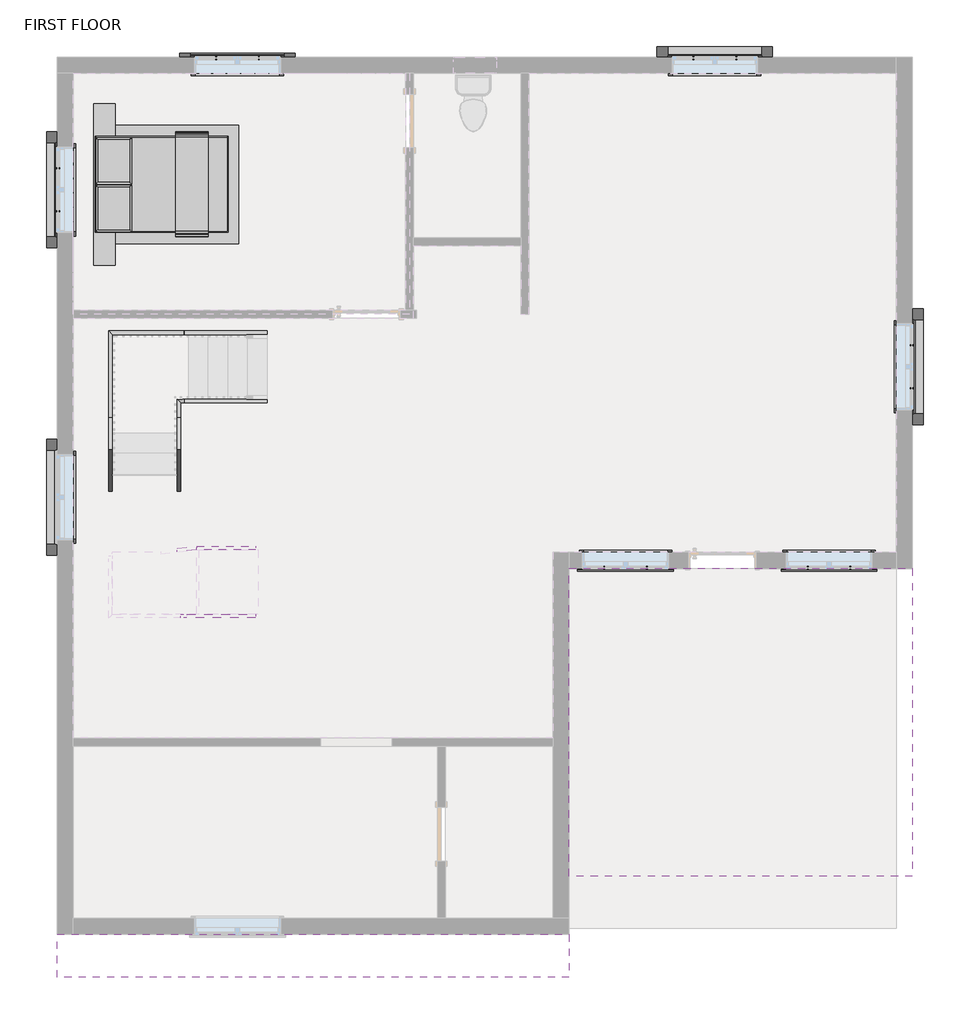
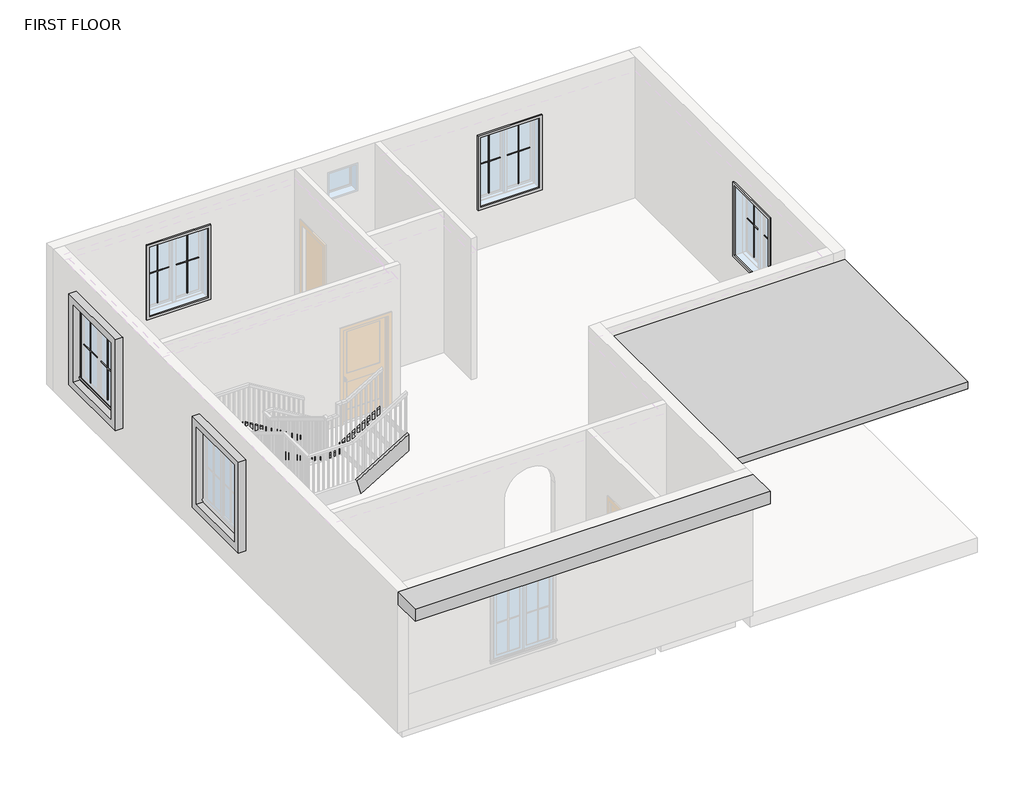
# One storey, part 4 of 4: 33 proxies, 10 members.
"""IFC4 building model written with IfcOpenShell, lengths in millimetres."""

from ifc_helpers import new_model, si_unit, frame, origin, place, context, project, spatial, polyline, outline, extrude, faceted_brep, transform, mapped, element, save
from components import bed_6467_bed_6467_bd858abb, generic_models_1_generic_models_1_44a9a556, generic_models_12_generic_models_12_6289c3a4, generic_models_14_generic_models_14_14abf339, generic_models_18_generic_models_18_24b474a2, generic_models_8_generic_models_8_5a9fc4db, muntin_pattern_2x2_muntin_pattern_2x2_6dad3731, muntin_pattern_2x2_muntin_pattern_2x2_a30a3345, trim_window_exterior_flat_with_sill_92b9b949, trim_window_interior_flat_picture_frame_3bb882cf

model = new_model("IFC4")

# Units and contexts
model_context = context("Model", 3, world=origin())
ifc_project = project(units=[si_unit("LENGTHUNIT", "METRE", prefix="MILLI")], contexts=[model_context])

# Site, building, storey
site = spatial("IfcSite", under=ifc_project)
building = spatial("IfcBuilding", under=site)
storey = spatial("IfcBuildingStorey", under=building, Name="FIRST FLOOR", Elevation=3352.8)

# Proxies
placement = place(None, origin())
bed_6467_bed_6467_shape = bed_6467_bed_6467_bd858abb(model_context)
element("IfcBuildingElementProxy", 1, Name="BED_6467 : BED_6467", ObjectType="BED_6467 : BED_6467", at=placement, inside=storey, context=model_context, shape_type="MappedRepresentation", body=[
    mapped(bed_6467_bed_6467_shape, transform((-10713.6322298, 3200.7413457, 3352.8), x_axis=(0.0, 1.0, 0.0), y_axis=(-1.0, 0.0, 0.0), z_axis=(0.0, 0.0, 1.0))),
])
generic_models_1_generic_models_1_shape = generic_models_1_generic_models_1_44a9a556(model_context)
element("IfcBuildingElementProxy", 2, Name="Generic Models 1 : Generic Models 1", ObjectType="Generic Models 1 : Generic Models 1", at=placement, inside=storey, context=model_context, shape_type="MappedRepresentation", body=[
    mapped(generic_models_1_generic_models_1_shape, transform((0.0, 0.0, 0.0), x_axis=(1.0, 0.0, 0.0), y_axis=(0.0, 1.0, 0.0), z_axis=(0.0, 0.0, 1.0))),
])
generic_models_12_generic_models_12_shape = generic_models_12_generic_models_12_6289c3a4(model_context)
element("IfcBuildingElementProxy", 3, Name="Generic Models 13 : Generic Models 12", ObjectType="Generic Models 13 : Generic Models 12", at=placement, inside=storey, context=model_context, shape_type="MappedRepresentation", body=[
    mapped(generic_models_12_generic_models_12_shape, transform((0.0, 0.0, 3048.0), x_axis=(1.0, 0.0, 0.0), y_axis=(0.0, 1.0, 0.0), z_axis=(0.0, 0.0, 1.0))),
])
generic_models_14_generic_models_14_shape = generic_models_14_generic_models_14_14abf339(model_context)
element("IfcBuildingElementProxy", 4, Name="Generic Models 14 : Generic Models 14", ObjectType="Generic Models 14 : Generic Models 14", at=placement, inside=storey, context=model_context, shape_type="MappedRepresentation", body=[
    mapped(generic_models_14_generic_models_14_shape, transform((0.0, 0.0, 25.4), x_axis=(1.0, 0.0, 0.0), y_axis=(0.0, 1.0, 0.0), z_axis=(0.0, 0.0, 1.0))),
])
element("IfcBuildingElementProxy", 5, Name="Generic Models 15 : Generic Models 14", ObjectType="Generic Models 15 : Generic Models 14", at=placement, inside=storey, context=model_context, shape_type="MappedRepresentation", body=[
    mapped(generic_models_14_generic_models_14_shape, transform((-6762.75, -95.25, 0.0), x_axis=(1.0, 0.0, 0.0), y_axis=(0.0, 1.0, 0.0), z_axis=(0.0, 0.0, 1.0))),
])
generic_models_18_generic_models_18_shape = generic_models_18_generic_models_18_24b474a2(model_context)
element("IfcBuildingElementProxy", 6, Name="Generic Models 18 : Generic Models 18", ObjectType="Generic Models 18 : Generic Models 18", at=placement, inside=storey, context=model_context, shape_type="MappedRepresentation", body=[
    mapped(generic_models_18_generic_models_18_shape, transform((0.0, 0.0, 0.0), x_axis=(1.0, 0.0, 0.0), y_axis=(0.0, 1.0, 0.0), z_axis=(0.0, 0.0, 1.0))),
])
element("IfcBuildingElementProxy", 7, Name="Generic Models 19 : Generic Models 18", ObjectType="Generic Models 19 : Generic Models 18", at=placement, inside=storey, context=model_context, shape_type="MappedRepresentation", body=[
    mapped(generic_models_18_generic_models_18_shape, transform((0.0, -4352.925, 0.0), x_axis=(1.0, 0.0, 0.0), y_axis=(0.0, 1.0, 0.0), z_axis=(0.0, 0.0, 1.0))),
])
generic_models_8_generic_models_8_shape = generic_models_8_generic_models_8_5a9fc4db(model_context)
element("IfcBuildingElementProxy", 8, Name="Generic Models 8 : Generic Models 8", ObjectType="Generic Models 8 : Generic Models 8", at=placement, inside=storey, context=model_context, shape_type="MappedRepresentation", body=[
    mapped(generic_models_8_generic_models_8_shape, transform((0.0, 0.0, 0.0), x_axis=(1.0, 0.0, 0.0), y_axis=(0.0, 1.0, 0.0), z_axis=(0.0, 0.0, 1.0))),
])
muntin_pattern_2x2_muntin_pattern_2x2_shape = muntin_pattern_2x2_muntin_pattern_2x2_6dad3731(model_context)
element("IfcBuildingElementProxy", 9, Name="Muntin Pattern_2x2 : Muntin Pattern_2x2", ObjectType="Muntin Pattern_2x2 : Muntin Pattern_2x2", at=placement, inside=storey, context=model_context, shape_type="MappedRepresentation", body=[
    mapped(muntin_pattern_2x2_muntin_pattern_2x2_shape, transform((-811.7461008, -2258.8594117, 4337.05), x_axis=(-1.0, 0.0, 0.0), y_axis=(0.0, -1.0, 0.0), z_axis=(0.0, 0.0, 1.0))),
])
element("IfcBuildingElementProxy", 10, Name="Muntin Pattern_2x2 : Muntin Pattern_2x2", ObjectType="Muntin Pattern_2x2 : Muntin Pattern_2x2", at=placement, inside=storey, context=model_context, shape_type="MappedRepresentation", body=[
    mapped(muntin_pattern_2x2_muntin_pattern_2x2_shape, transform((-3694.6461008, -2258.8594117, 4337.05), x_axis=(-1.0, 0.0, 0.0), y_axis=(0.0, -1.0, 0.0), z_axis=(0.0, 0.0, 1.0))),
])
element("IfcBuildingElementProxy", 11, Name="Muntin Pattern_2x2 : Muntin Pattern_2x2", ObjectType="Muntin Pattern_2x2 : Muntin Pattern_2x2", at=placement, inside=storey, context=model_context, shape_type="MappedRepresentation", body=[
    mapped(muntin_pattern_2x2_muntin_pattern_2x2_shape, transform((56.6163992, 892.3280883, 4337.05), x_axis=(0.0, -1.0, 0.0), y_axis=(1.0, 0.0, 0.0), z_axis=(0.0, 0.0, 1.0))),
])
element("IfcBuildingElementProxy", 12, Name="Muntin Pattern_2x2 : Muntin Pattern_2x2", ObjectType="Muntin Pattern_2x2 : Muntin Pattern_2x2", at=placement, inside=storey, context=model_context, shape_type="MappedRepresentation", body=[
    mapped(muntin_pattern_2x2_muntin_pattern_2x2_shape, transform((-9800.1711008, 4961.0905883, 4337.05), x_axis=(1.0, 0.0, 0.0), y_axis=(0.0, 1.0, 0.0), z_axis=(0.0, 0.0, 1.0))),
])
element("IfcBuildingElementProxy", 13, Name="Muntin Pattern_2x2 : Muntin Pattern_2x2", ObjectType="Muntin Pattern_2x2 : Muntin Pattern_2x2", at=placement, inside=storey, context=model_context, shape_type="MappedRepresentation", body=[
    mapped(muntin_pattern_2x2_muntin_pattern_2x2_shape, transform((-12040.1336008, 2790.9780883, 4337.05), x_axis=(0.0, 1.0, 0.0), y_axis=(-1.0, 0.0, 0.0), z_axis=(0.0, 0.0, 1.0))),
])
element("IfcBuildingElementProxy", 14, Name="Muntin Pattern_2x2 : Muntin Pattern_2x2", ObjectType="Muntin Pattern_2x2 : Muntin Pattern_2x2", at=placement, inside=storey, context=model_context, shape_type="MappedRepresentation", body=[
    mapped(muntin_pattern_2x2_muntin_pattern_2x2_shape, transform((-3037.4211008, 4961.0905883, 4337.05), x_axis=(1.0, 0.0, 0.0), y_axis=(0.0, 1.0, 0.0), z_axis=(0.0, 0.0, 1.0))),
])
muntin_pattern_2x2_muntin_pattern_2x2_2_shape = muntin_pattern_2x2_muntin_pattern_2x2_a30a3345(model_context)
element("IfcBuildingElementProxy", 15, Name="Muntin Pattern_2x2 : Muntin Pattern_2x2", ObjectType="Muntin Pattern_2x2 : Muntin Pattern_2x2", at=placement, inside=storey, context=model_context, shape_type="MappedRepresentation", body=[
    mapped(muntin_pattern_2x2_muntin_pattern_2x2_2_shape, transform((-1418.1711008, -2258.8594117, 4337.05), x_axis=(1.0, 0.0, 0.0), y_axis=(0.0, 1.0, 0.0), z_axis=(0.0, 0.0, 1.0))),
])
element("IfcBuildingElementProxy", 16, Name="Muntin Pattern_2x2 : Muntin Pattern_2x2", ObjectType="Muntin Pattern_2x2 : Muntin Pattern_2x2", at=placement, inside=storey, context=model_context, shape_type="MappedRepresentation", body=[
    mapped(muntin_pattern_2x2_muntin_pattern_2x2_2_shape, transform((-4301.0711008, -2258.8594117, 4337.05), x_axis=(1.0, 0.0, 0.0), y_axis=(0.0, 1.0, 0.0), z_axis=(0.0, 0.0, 1.0))),
])
element("IfcBuildingElementProxy", 17, Name="Muntin Pattern_2x2 : Muntin Pattern_2x2", ObjectType="Muntin Pattern_2x2 : Muntin Pattern_2x2", at=placement, inside=storey, context=model_context, shape_type="MappedRepresentation", body=[
    mapped(muntin_pattern_2x2_muntin_pattern_2x2_2_shape, transform((56.6163992, 285.9030883, 4337.05), x_axis=(0.0, 1.0, 0.0), y_axis=(-1.0, 0.0, 0.0), z_axis=(0.0, 0.0, 1.0))),
])
element("IfcBuildingElementProxy", 18, Name="Muntin Pattern_2x2 : Muntin Pattern_2x2", ObjectType="Muntin Pattern_2x2 : Muntin Pattern_2x2", at=placement, inside=storey, context=model_context, shape_type="MappedRepresentation", body=[
    mapped(muntin_pattern_2x2_muntin_pattern_2x2_2_shape, transform((-9193.7461008, 4961.0905883, 4337.05), x_axis=(-1.0, 0.0, 0.0), y_axis=(0.0, -1.0, 0.0), z_axis=(0.0, 0.0, 1.0))),
])
element("IfcBuildingElementProxy", 19, Name="Muntin Pattern_2x2 : Muntin Pattern_2x2", ObjectType="Muntin Pattern_2x2 : Muntin Pattern_2x2", at=placement, inside=storey, context=model_context, shape_type="MappedRepresentation", body=[
    mapped(muntin_pattern_2x2_muntin_pattern_2x2_2_shape, transform((-12040.1336008, 3397.4030883, 4337.05), x_axis=(0.0, -1.0, 0.0), y_axis=(1.0, 0.0, 0.0), z_axis=(0.0, 0.0, 1.0))),
])
element("IfcBuildingElementProxy", 20, Name="Muntin Pattern_2x2 : Muntin Pattern_2x2", ObjectType="Muntin Pattern_2x2 : Muntin Pattern_2x2", at=placement, inside=storey, context=model_context, shape_type="MappedRepresentation", body=[
    mapped(muntin_pattern_2x2_muntin_pattern_2x2_2_shape, transform((-2430.9961008, 4961.0905883, 4337.05), x_axis=(-1.0, 0.0, 0.0), y_axis=(0.0, -1.0, 0.0), z_axis=(0.0, 0.0, 1.0))),
])
trim_window_exterior_flat_with_sill_shape = trim_window_exterior_flat_with_sill_92b9b949(model_context)
element("IfcBuildingElementProxy", 21, Name="Trim-Window-Exterior-Flat : with Sill", ObjectType="Trim-Window-Exterior-Flat : with Sill", at=placement, inside=storey, context=model_context, shape_type="MappedRepresentation", body=[
    mapped(trim_window_exterior_flat_with_sill_shape, transform((-1114.9586008, -2268.3844117, 5791.2), x_axis=(1.0, 0.0, 0.0), y_axis=(0.0, 0.0, 1.0), z_axis=(0.0, -1.0, 0.0))),
])
element("IfcBuildingElementProxy", 22, Name="Trim-Window-Exterior-Flat : with Sill", ObjectType="Trim-Window-Exterior-Flat : with Sill", at=placement, inside=storey, context=model_context, shape_type="MappedRepresentation", body=[
    mapped(trim_window_exterior_flat_with_sill_shape, transform((-3997.8586008, -2268.3844117, 5791.2), x_axis=(1.0, 0.0, 0.0), y_axis=(0.0, 0.0, 1.0), z_axis=(0.0, -1.0, 0.0))),
])
element("IfcBuildingElementProxy", 23, Name="Trim-Window-Exterior-Flat : with Sill", ObjectType="Trim-Window-Exterior-Flat : with Sill", at=placement, inside=storey, context=model_context, shape_type="MappedRepresentation", body=[
    mapped(trim_window_exterior_flat_with_sill_shape, transform((66.1413992, 589.1155883, 5791.2), x_axis=(0.0, 1.0, 0.0), y_axis=(0.0, 0.0, 1.0), z_axis=(1.0, 0.0, 0.0))),
])
element("IfcBuildingElementProxy", 24, Name="Trim-Window-Exterior-Flat : with Sill", ObjectType="Trim-Window-Exterior-Flat : with Sill", at=placement, inside=storey, context=model_context, shape_type="MappedRepresentation", body=[
    mapped(trim_window_exterior_flat_with_sill_shape, transform((-9496.9586008, 4970.6155883, 5791.2), x_axis=(-1.0, 0.0, 0.0), y_axis=(0.0, 0.0, 1.0), z_axis=(0.0, 1.0, 0.0))),
])
element("IfcBuildingElementProxy", 25, Name="Trim-Window-Exterior-Flat : with Sill", ObjectType="Trim-Window-Exterior-Flat : with Sill", at=placement, inside=storey, context=model_context, shape_type="MappedRepresentation", body=[
    mapped(trim_window_exterior_flat_with_sill_shape, transform((-12049.6586008, 3094.1905883, 5791.2), x_axis=(0.0, -1.0, 0.0), y_axis=(0.0, 0.0, 1.0), z_axis=(-1.0, 0.0, 0.0))),
])
element("IfcBuildingElementProxy", 26, Name="Trim-Window-Exterior-Flat : with Sill", ObjectType="Trim-Window-Exterior-Flat : with Sill", at=placement, inside=storey, context=model_context, shape_type="MappedRepresentation", body=[
    mapped(trim_window_exterior_flat_with_sill_shape, transform((-2734.2086008, 4970.6155883, 5791.2), x_axis=(-1.0, 0.0, 0.0), y_axis=(0.0, 0.0, 1.0), z_axis=(0.0, 1.0, 0.0))),
])
trim_window_interior_flat_picture_frame_shape = trim_window_interior_flat_picture_frame_3bb882cf(model_context)
element("IfcBuildingElementProxy", 27, Name="Trim-Window-Interior-Flat : Picture Frame", ObjectType="Trim-Window-Interior-Flat : Picture Frame", at=placement, inside=storey, context=model_context, shape_type="MappedRepresentation", body=[
    mapped(trim_window_interior_flat_picture_frame_shape, transform((-1114.9586008, -2039.7844117, 5791.2), x_axis=(-1.0, 0.0, 0.0), y_axis=(0.0, 0.0, 1.0), z_axis=(0.0, 1.0, 0.0))),
])
element("IfcBuildingElementProxy", 28, Name="Trim-Window-Interior-Flat : Picture Frame", ObjectType="Trim-Window-Interior-Flat : Picture Frame", at=placement, inside=storey, context=model_context, shape_type="MappedRepresentation", body=[
    mapped(trim_window_interior_flat_picture_frame_shape, transform((-3997.8586008, -2039.7844117, 5791.2), x_axis=(-1.0, 0.0, 0.0), y_axis=(0.0, 0.0, 1.0), z_axis=(0.0, 1.0, 0.0))),
])
element("IfcBuildingElementProxy", 29, Name="Trim-Window-Interior-Flat : Picture Frame", ObjectType="Trim-Window-Interior-Flat : Picture Frame", at=placement, inside=storey, context=model_context, shape_type="MappedRepresentation", body=[
    mapped(trim_window_interior_flat_picture_frame_shape, transform((-162.4586008, 589.1155883, 5791.2), x_axis=(0.0, -1.0, 0.0), y_axis=(0.0, 0.0, 1.0), z_axis=(-1.0, 0.0, 0.0))),
])
element("IfcBuildingElementProxy", 30, Name="Trim-Window-Interior-Flat : Picture Frame", ObjectType="Trim-Window-Interior-Flat : Picture Frame", at=placement, inside=storey, context=model_context, shape_type="MappedRepresentation", body=[
    mapped(trim_window_interior_flat_picture_frame_shape, transform((-9496.9586008, 4742.0155883, 5791.2), x_axis=(1.0, 0.0, 0.0), y_axis=(0.0, 0.0, 1.0), z_axis=(0.0, -1.0, 0.0))),
])
element("IfcBuildingElementProxy", 31, Name="Trim-Window-Interior-Flat : Picture Frame", ObjectType="Trim-Window-Interior-Flat : Picture Frame", at=placement, inside=storey, context=model_context, shape_type="MappedRepresentation", body=[
    mapped(trim_window_interior_flat_picture_frame_shape, transform((-11821.0586008, 3094.1905883, 5791.2), x_axis=(0.0, 1.0, 0.0), y_axis=(0.0, 0.0, 1.0), z_axis=(1.0, 0.0, 0.0))),
])
element("IfcBuildingElementProxy", 32, Name="Trim-Window-Interior-Flat : Picture Frame", ObjectType="Trim-Window-Interior-Flat : Picture Frame", at=placement, inside=storey, context=model_context, shape_type="MappedRepresentation", body=[
    mapped(trim_window_interior_flat_picture_frame_shape, transform((-11821.0586008, -1258.7344117, 5791.2), x_axis=(0.0, 1.0, 0.0), y_axis=(0.0, 0.0, 1.0), z_axis=(1.0, 0.0, 0.0))),
])
element("IfcBuildingElementProxy", 33, Name="Trim-Window-Interior-Flat : Picture Frame", ObjectType="Trim-Window-Interior-Flat : Picture Frame", at=placement, inside=storey, context=model_context, shape_type="MappedRepresentation", body=[
    mapped(trim_window_interior_flat_picture_frame_shape, transform((-2734.2086008, 4742.0155883, 5791.2), x_axis=(1.0, 0.0, 0.0), y_axis=(0.0, 0.0, 1.0), z_axis=(0.0, -1.0, 0.0))),
])

# Members
element("IfcMember", 34, ObjectType="Stringer - 2\" Width", at=placement, inside=storey, context=model_context, shape_type="SweptSolid", body=[
    extrude(outline(polyline([(3352.8, -9079.7156858), (3564.914512, -9079.7156858), (4275.6666667, -10252.4567411), (3970.8666667, -10337.6111976), (3352.8, -9317.8011976), (3352.8, -9079.7156858)])), frame((0.0, 79.9115003, 0.0), z_axis=(0.0, 1.0, 0.0), x_axis=(0.0, 0.0, 1.0)), (0.0, 0.0, 1.0), 50.8),
])
element("IfcMember", 35, ObjectType="Stringer - 2\" Width", at=placement, inside=storey, context=model_context, shape_type="SweptSolid", body=[
    extrude(outline(polyline([(3352.8, -9079.7156858), (3564.914512, -9079.7156858), (4275.6666667, -10252.4567411), (3970.8666667, -10337.6111976), (3352.8, -9317.8011976), (3352.8, -9079.7156858)])), frame((0.0, 1045.1115003, 0.0), z_axis=(0.0, 1.0, 0.0), x_axis=(0.0, 0.0, 1.0)), (0.0, 0.0, 1.0), 50.8),
])
element("IfcMember", 36, ObjectType="Stringer - 2\" Width", at=placement, inside=storey, context=model_context, shape_type="Brep", body=[
    faceted_brep([(-10302.9522729, -132.1404207, 4275.6666667), (-10353.7522729, -132.1404207, 4275.6666667), (-10353.7522729, -1981.6853298, 5396.6029752), (-10302.9522729, -1976.0280655, 5393.1743302), (-10302.9522729, -217.2948772, 3970.8666667), (-10302.9522729, -1976.0280655, 5036.7655687), (-10353.7522729, -217.2948772, 3970.8666667), (-10353.7522729, -1981.6853298, 5040.1942137)], [[[0, 1, 2, 3]], [[4, 0, 3, 5]], [[6, 4, 5, 7]], [[1, 6, 7, 2]], [[1, 0, 4, 6]], [[2, 7, 5, 3]]]),
])
element("IfcMember", 37, ObjectType="Stringer - 2\" Width", at=placement, inside=storey, context=model_context, shape_type="SweptSolid", body=[
    extrude(outline(polyline([(-132.1404207, 4275.6666667), (-217.2948772, 3970.8666667), (-2173.0948772, 5156.2), (-2087.9404207, 5461.0), (-132.1404207, 4275.6666667)])), frame((-11318.9522729, 0.0, 0.0), z_axis=(1.0, 0.0, 0.0), x_axis=(0.0, 1.0, 0.0)), (0.0, 0.0, 1.0), 50.8),
])
element("IfcMember", 38, ObjectType="Stringer - 2\" Width", at=placement, inside=storey, context=model_context, shape_type="Brep", body=[
    faceted_brep([(-10353.7522729, -132.1404207, 4275.6666667), (-10302.9522729, -132.1404207, 4275.6666667), (-10302.9522729, 79.9115003, 4275.6666667), (-10353.7522729, 130.7115003, 4275.6666667), (-10353.7522729, -217.2948772, 3970.8666667), (-10353.7522729, 130.7115003, 3970.8666667), (-10302.9522729, -217.2948772, 3970.8666667), (-10302.9522729, 79.9115003, 3970.8666667)], [[[0, 1, 2, 3]], [[4, 0, 3, 5]], [[6, 4, 5, 7]], [[1, 6, 7, 2]], [[1, 0, 4, 6]], [[2, 7, 5, 3]]]),
])
element("IfcMember", 39, ObjectType="Stringer - 2\" Width", at=placement, inside=storey, context=model_context, shape_type="Brep", body=[
    faceted_brep([(-10252.4567411, 1045.1115003, 4275.6666667), (-10252.4567411, 1095.9115003, 4275.6666667), (-11318.9522729, 1095.9115003, 4275.6666667), (-11268.1522729, 1045.1115003, 4275.6666667), (-10337.6111976, 1045.1115003, 3970.8666667), (-11268.1522729, 1045.1115003, 3970.8666667), (-10337.6111976, 1095.9115003, 3970.8666667), (-11318.9522729, 1095.9115003, 3970.8666667)], [[[0, 1, 2, 3]], [[4, 0, 3, 5]], [[6, 4, 5, 7]], [[1, 6, 7, 2]], [[1, 0, 4, 6]], [[2, 7, 5, 3]]]),
])
element("IfcMember", 40, ObjectType="Stringer - 2\" Width", at=placement, inside=storey, context=model_context, shape_type="Brep", body=[
    faceted_brep([(-11268.1522729, 1045.1115003, 4275.6666667), (-11318.9522729, 1095.9115003, 4275.6666667), (-11318.9522729, -132.1404207, 4275.6666667), (-11268.1522729, -132.1404207, 4275.6666667), (-11268.1522729, 1045.1115003, 3970.8666667), (-11268.1522729, -217.2948772, 3970.8666667), (-11318.9522729, 1095.9115003, 3970.8666667), (-11318.9522729, -217.2948772, 3970.8666667)], [[[0, 1, 2, 3]], [[4, 0, 3, 5]], [[6, 4, 5, 7]], [[1, 6, 7, 2]], [[1, 0, 4, 6]], [[2, 7, 5, 3]]]),
])
element("IfcMember", 41, ObjectType="Stringer - 2\" Width", at=placement, inside=storey, context=model_context, shape_type="SweptSolid", body=[
    extrude(outline(polyline([(5596.914512, -10074.3522729), (5240.5057504, -10074.3522729), (5748.5057504, -9236.1522729), (6104.914512, -9236.1522729), (5596.914512, -10074.3522729)])), frame((0.0, -2001.6844117, 0.0), z_axis=(0.0, 1.0, 0.0), x_axis=(0.0, 0.0, 1.0)), (0.0, 0.0, 1.0), 50.8),
])
element("IfcMember", 42, ObjectType="Stringer - 2\" Width", at=placement, inside=storey, context=model_context, shape_type="SweptSolid", body=[
    extrude(outline(polyline([(5461.0, -10298.6112176), (5156.2, -10213.4567611), (5748.5057504, -9236.1522729), (6104.914512, -9236.1522729), (5461.0, -10298.6112176)])), frame((0.0, -2966.8844117, 0.0), z_axis=(0.0, 1.0, 0.0), x_axis=(0.0, 0.0, 1.0)), (0.0, 0.0, 1.0), 50.8),
])
element("IfcMember", 43, ObjectType="Stringer - 2\" Width", at=placement, inside=storey, context=model_context, shape_type="SweptSolid", body=[
    extrude(outline(polyline([(-10074.3522729, -1950.570376), (-10074.3522729, -2001.6844117), (-10353.7522729, -2032.7993654), (-10353.7522729, -1981.6853298), (-10074.3522729, -1950.570376)])), frame((0.0, 0.0, 5156.2), z_axis=(0.0, 0.0, 1.0), x_axis=(1.0, 0.0, 0.0)), (0.0, 0.0, 1.0), 304.8),
])

save(model, "model.ifc")

# Revit data of these elements
# Type "BED_6467 : BED_6467"
#   Sheets [instance default] = Sheets
#   Pillow Set 2 [instance default] = Pillow 2
#   Pillow Set 1 [instance default] = Pillow 1
#   FRAME [instance default] = FRAME
#   Default Elevation = 0
# Type "Muntin Pattern_2x2 : Muntin Pattern_2x2"
#   Width [instance default] = 4' - 0"
#   Thickness = 0' - 0 1/2"
#   Height [instance default] = 4' - 0"
#   Distance = 0' - 0 3/4"
#   Interior Material [instance default] = none
#   Exterior Material [instance default] = none
#   Default Elevation = 0
# Type "Trim-Window-Exterior-Flat : with Sill"
#   Trim Width = 0' - 2 1/4"
#   Trim Thickness_Picture Frame = 0' - 1 1/4"
#   Trim Thickness_with Sill = 0' - 0 3/4"
#   Sill Thickness = 0' - 1 1/4"
#   Opening Width [instance default] = 2' - 0"
#   Opening Height [instance default] = 3' - 0"
#   Default Elevation = 4' - 0"
#   Sill = yes
#   Picture Frame = no
#   Trim Material [instance default] = none
# Type "Trim-Window-Interior-Flat : Picture Frame"
#   Trim Thickness_Picture Frame = 0' - 1 1/4"
#   Trim Width = 0' - 2 1/4"
#   Trim Thickness_with Sill = 0' - 0 3/4"
#   Sill Thickness = 0' - 1 1/4"
#   Opening Width [instance default] = 2' - 0"
#   Opening Height [instance default] = 3' - 0"
#   Default Elevation = 4' - 0"
#   Sill = no
#   Picture Frame = yes
#   Trim Material [instance default] = none
# Element 1 (IfcBuildingElementProxy, "BED_6467 : BED_6467")
#   Sheets = Sheets
#   Pillow Set 2 = Pillow 2
#   Pillow Set 1 = Pillow 1
#   FRAME = FRAME
#   Phase Created = New Construction
#   Materials on its faces: "FRAME", "Pillow 1", "Pillow 2", "Sheets"
# Element 2 (IfcBuildingElementProxy, "Generic Models 1 : Generic Models 1")
#   Phase Created = New Construction
#   Materials on its faces: "Clad - White"
# Element 3 (IfcBuildingElementProxy, "Generic Models 13 : Generic Models 12")
#   Phase Created = New Construction
#   Materials on its faces: "feature frame"
# Element 4 (IfcBuildingElementProxy, "Generic Models 14 : Generic Models 14")
#   Phase Created = New Construction
#   Materials on its faces: "feature frame"
# Element 5 (IfcBuildingElementProxy, "Generic Models 15 : Generic Models 14")
#   Phase Created = New Construction
#   Materials on its faces: "feature frame"
# Element 6 (IfcBuildingElementProxy, "Generic Models 18 : Generic Models 18")
#   Phase Created = New Construction
#   Materials on its faces: "feature frame"
# Element 7 (IfcBuildingElementProxy, "Generic Models 19 : Generic Models 18")
#   Phase Created = New Construction
#   Materials on its faces: "feature frame"
# Element 8 (IfcBuildingElementProxy, "Generic Models 8 : Generic Models 8")
#   Phase Created = New Construction
#   Materials on its faces: "wood ceiling"
# Elements 9, 10, 11, 12, 13, 14, 15, 16, 17, 18, 19, 20 (IfcBuildingElementProxy, "Muntin Pattern_2x2 : Muntin Pattern_2x2")
#   Width = 1' - 6 5/8"
#   Height = 4' - 6 1/2"
#   Interior Material = Wood - Stained
#   Exterior Material = BLACK MATERIAL
#   Phase Created = New Construction
#   Materials on its faces: "BLACK MATERIAL", "Wood - Stained"
# Elements 21, 22, 23, 24, 25, 26 (IfcBuildingElementProxy, "Trim-Window-Exterior-Flat : with Sill")
#   Opening Width = 4' - 0"
#   Opening Height = 5' - 0"
#   Trim Material = BLACK MATERIAL
#   Phase Created = New Construction
#   Materials on its faces: "BLACK MATERIAL"
# Elements 27, 28, 29, 30, 31, 32, 33 (IfcBuildingElementProxy, "Trim-Window-Interior-Flat : Picture Frame")
#   Opening Width = 4' - 0"
#   Opening Height = 5' - 0"
#   Trim Material = Wood - Stained
#   Phase Created = New Construction
#   Materials on its faces: "Wood - Stained"
# Elements 34, 35, 36, 37, 38, 39, 40, 41, 42, 43 (IfcMember, "Stringer - 2\" Width")
#   Phase Created = New Construction
# Materials
#   "Sheets": class "Fabric", colour RGB 255 255 255, transparency 0
#   "Pillow 2": class "Fabric", colour RGB 255 255 255, transparency 0
#   "Pillow 1": class "Fabric", colour RGB 0 64 128, transparency 0
#   "FRAME": class "Paint", colour RGB 58 58 58, transparency 0
#   "Clad - White": class "Wood", colour RGB 242 242 238, transparency 0, Cost = 0
#   "feature frame": class "Generic", colour RGB 120 120 120, transparency 0, Cost = 0
#   "wood ceiling": class "Generic", colour RGB 120 120 120, transparency 0, Cost = 0
#   "BLACK MATERIAL": class "Generic", colour RGB 120 120 120, transparency 0, Cost = 0
#   "Wood - Stained": class "Wood", colour RGB 224 178 126, transparency 0, Cost = 0
